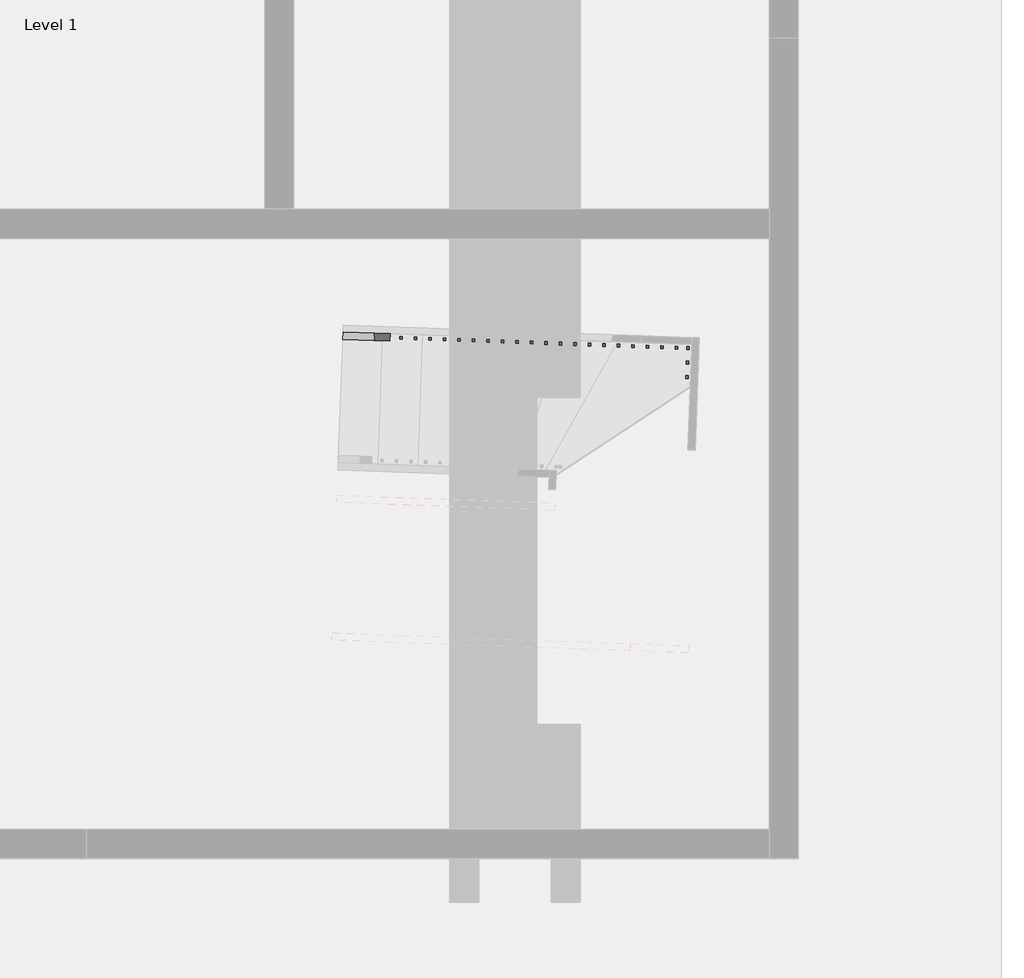
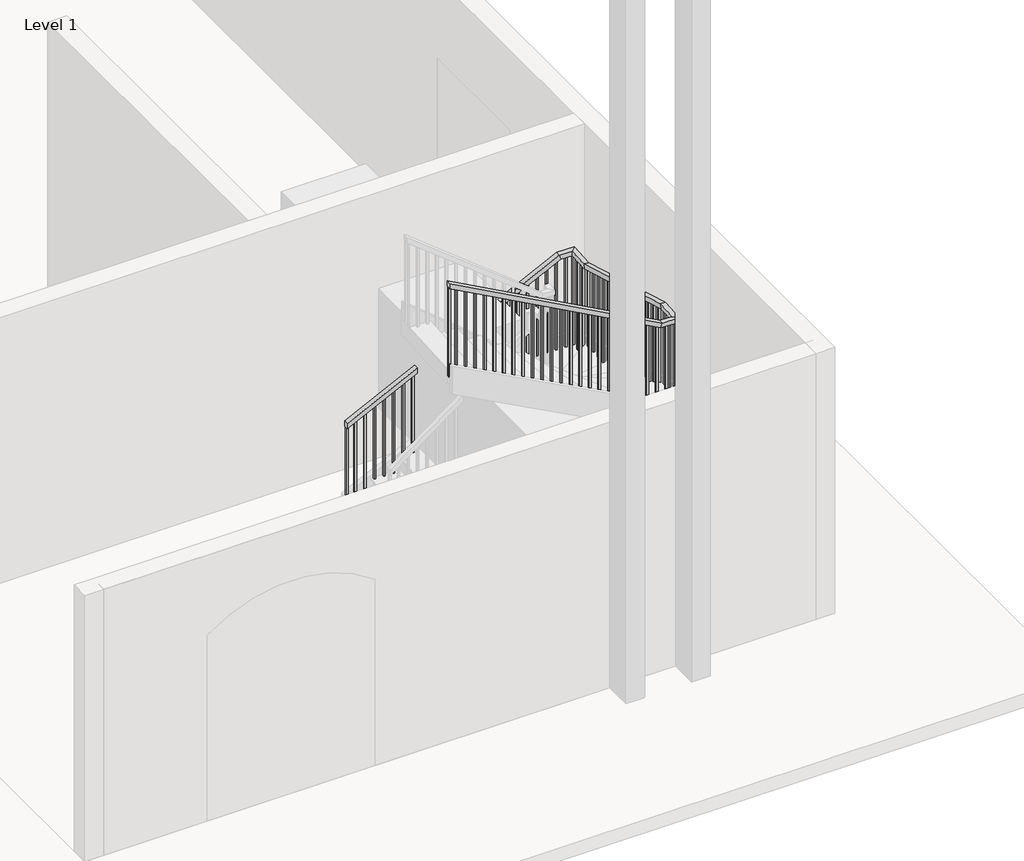
# One storey, part 3 of 4: 1 railing.
"""IFC4 building model written with IfcOpenShell, lengths in millimetres."""

from ifc_helpers import new_model, si_unit, frame, origin, place, context, project, spatial, polyline, outline, extrude, faceted_brep, element, save

model = new_model("IFC4")

# Units and contexts
model_context = context("Model", 3, world=origin())
ifc_project = project(units=[si_unit("LENGTHUNIT", "METRE", prefix="MILLI")], contexts=[model_context])

# Site, building, storey
site = spatial("IfcSite", under=ifc_project)
building = spatial("IfcBuilding", under=site)
storey = spatial("IfcBuildingStorey", under=building, Name="Level 1", Elevation=0.0)

# Railing
placement = place(None, origin())
element("IfcRailing", 1, ObjectType="Handrail - Rectangular", at=placement, inside=storey, context=model_context, shape_type="SolidModel", body=[
    faceted_brep([(-10006.394185, -363.3128759, 1083.7333333), (-10006.394185, -363.3128759, 1026.2742652), (-10008.220866, -414.0800231, 1026.2742652), (-10008.220866, -414.0800231, 1083.7333333), (-7750.1292126, -444.496803, 2277.0239201), (-7737.5382959, -444.9498438, 2226.2239201), (-7739.364977, -495.716991, 2226.2239201), (-7751.9558936, -495.2639503, 2277.0239201), (-7565.8418401, -451.1277497, 2277.0239201), (-7565.8418401, -451.1277497, 2226.2239201), (-7618.4356683, -500.0682159, 2226.2239201), (-7618.4356683, -500.0682159, 2277.0239201), (-7576.1730834, -738.2538248, 2277.0239201), (-7576.4589725, -746.1992592, 2226.2239201), (-7627.2261197, -744.3725782, 2226.2239201), (-7626.9402306, -736.4271438, 2277.0239201), (-7631.3178587, -2270.838284, 2769.1094132), (-7631.6037478, -2278.7837184, 2718.3094132), (-7682.370895, -2276.9570374, 2718.3094132), (-7682.0850059, -2269.011603, 2769.1094132), (-7641.649102, -2557.9643591, 2769.1094132), (-7641.649102, -2557.9643591, 2718.3094132), (-7690.5895682, -2505.3705309, 2718.3094132), (-7690.5895682, -2505.3705309, 2769.1094132), (-7825.9364745, -2551.3334125, 2769.1094132), (-7838.5273911, -2550.8803717, 2718.3094132), (-7836.7007101, -2500.1132245, 2718.3094132), (-7824.1097935, -2500.5662653, 2769.1094132), (-10082.2014469, -2470.1494854, 3962.4), (-10080.3747659, -2419.3823382, 3962.4), (-10080.3747659, -2419.3823382, 3904.9409318), (-10082.2014469, -2470.1494854, 3904.9409318)], [[[0, 1, 2, 3]], [[1, 0, 4, 5]], [[2, 1, 5, 6]], [[3, 2, 6, 7]], [[0, 3, 7, 4]], [[5, 4, 8, 9]], [[6, 5, 9, 10]], [[7, 6, 10, 11]], [[4, 7, 11, 8]], [[9, 8, 12, 13]], [[10, 9, 13, 14]], [[11, 10, 14, 15]], [[8, 11, 15, 12]], [[13, 12, 16, 17]], [[14, 13, 17, 18]], [[15, 14, 18, 19]], [[12, 15, 19, 16]], [[17, 16, 20, 21]], [[18, 17, 21, 22]], [[19, 18, 22, 23]], [[16, 19, 23, 20]], [[21, 20, 24, 25]], [[22, 21, 25, 26]], [[23, 22, 26, 27]], [[20, 23, 27, 24]], [[28, 29, 30, 31]], [[25, 24, 28, 31]], [[26, 25, 31, 30]], [[27, 26, 30, 29]], [[24, 27, 29, 28]]]),
    extrude(outline(polyline([(223.5656878, 19.05), (1212.6274313, 19.05), (1212.6274313, 0.0), (233.6343122, 0.0), (223.5656878, 19.05)])), frame((-9992.2317697, -2457.5014613, 4091.294098), z_axis=(0.035958287618052934, 0.9993532916599503, 0.0), x_axis=(0.0, 0.0, -1.0)), (0.0, 0.0, 1.0), 19.05),
    extrude(outline(polyline([(223.5656878, 19.05), (1158.9281011, 19.05), (1158.9281011, 0.0), (233.6343122, 0.0), (223.5656878, 19.05)])), frame((-9890.6974752, -2461.1548233, 4037.5947678), z_axis=(0.035958287618052934, 0.9993532916599503, 0.0), x_axis=(0.0, 0.0, -1.0)), (0.0, 0.0, 1.0), 19.05),
    extrude(outline(polyline([(223.5656878, 19.05), (1274.5621043, 19.05), (1274.5621043, 0.0), (233.6343122, 0.0), (223.5656878, 19.05)])), frame((-9789.1631808, -2464.8081854, 3983.8954376), z_axis=(0.035958287618052934, 0.9993532916599503, 0.0), x_axis=(0.0, 0.0, -1.0)), (0.0, 0.0, 1.0), 19.05),
    extrude(outline(polyline([(223.5656878, 19.05), (1220.8627741, 19.05), (1220.8627741, 0.0), (233.6343122, 0.0), (223.5656878, 19.05)])), frame((-9687.6288864, -2468.4615474, 3930.1961074), z_axis=(0.035958287618052934, 0.9993532916599503, 0.0), x_axis=(0.0, 0.0, -1.0)), (0.0, 0.0, 1.0), 19.05),
    extrude(outline(polyline([(223.5656878, 19.05), (1167.1634439, 19.05), (1167.1634439, 0.0), (233.6343122, 0.0), (223.5656878, 19.05)])), frame((-9586.0945919, -2472.1149094, 3876.4967772), z_axis=(0.035958287618052934, 0.9993532916599503, 0.0), x_axis=(0.0, 0.0, -1.0)), (0.0, 0.0, 1.0), 19.05),
    extrude(outline(polyline([(223.5656878, 19.05), (1282.797447, 19.05), (1282.797447, 0.0), (233.6343122, 0.0), (223.5656878, 19.05)])), frame((-9484.5602975, -2475.7682714, 3822.797447), z_axis=(0.035958287618052934, 0.9993532916599503, 0.0), x_axis=(0.0, 0.0, -1.0)), (0.0, 0.0, 1.0), 19.05),
    extrude(outline(polyline([(223.5656878, 19.05), (1229.0981168, 19.05), (1229.0981168, 0.0), (233.6343122, 0.0), (223.5656878, 19.05)])), frame((-9383.0260031, -2479.4216334, 3769.0981168), z_axis=(0.035958287618052934, 0.9993532916599503, 0.0), x_axis=(0.0, 0.0, -1.0)), (0.0, 0.0, 1.0), 19.05),
    extrude(outline(polyline([(223.5656878, 19.05), (1175.3987866, 19.05), (1175.3987866, 0.0), (233.6343122, 0.0), (223.5656878, 19.05)])), frame((-9281.4917086, -2483.0749955, 3715.3987866), z_axis=(0.035958287618052934, 0.9993532916599503, 0.0), x_axis=(0.0, 0.0, -1.0)), (0.0, 0.0, 1.0), 19.05),
    extrude(outline(polyline([(223.5656878, 19.05), (1291.0327897, 19.05), (1291.0327897, 0.0), (233.6343122, 0.0), (223.5656878, 19.05)])), frame((-9179.9574142, -2486.7283575, 3661.6994564), z_axis=(0.035958287618052934, 0.9993532916599503, 0.0), x_axis=(0.0, 0.0, -1.0)), (0.0, 0.0, 1.0), 19.05),
    extrude(outline(polyline([(223.5656878, 19.05), (1237.3334595, 19.05), (1237.3334595, 0.0), (233.6343122, 0.0), (223.5656878, 19.05)])), frame((-9078.4231198, -2490.3817195, 3608.0001262), z_axis=(0.035958287618052934, 0.9993532916599503, 0.0), x_axis=(0.0, 0.0, -1.0)), (0.0, 0.0, 1.0), 19.05),
    extrude(outline(polyline([(223.5656878, 19.05), (1183.6341293, 19.05), (1183.6341293, 0.0), (233.6343122, 0.0), (223.5656878, 19.05)])), frame((-8976.8888253, -2494.0350815, 3554.300796), z_axis=(0.035958287618052934, 0.9993532916599503, 0.0), x_axis=(0.0, 0.0, -1.0)), (0.0, 0.0, 1.0), 19.05),
    extrude(outline(polyline([(223.5656878, 19.05), (1299.2681325, 19.05), (1299.2681325, 0.0), (233.6343122, 0.0), (223.5656878, 19.05)])), frame((-8875.3545309, -2497.6884436, 3500.6014658), z_axis=(0.035958287618052934, 0.9993532916599503, 0.0), x_axis=(0.0, 0.0, -1.0)), (0.0, 0.0, 1.0), 19.05),
    extrude(outline(polyline([(223.5656878, 19.05), (1245.5688023, 19.05), (1245.5688023, 0.0), (233.6343122, 0.0), (223.5656878, 19.05)])), frame((-8773.8202365, -2501.3418056, 3446.9021356), z_axis=(0.035958287618052934, 0.9993532916599503, 0.0), x_axis=(0.0, 0.0, -1.0)), (0.0, 0.0, 1.0), 19.05),
    extrude(outline(polyline([(223.5656878, 19.05), (1191.8694721, 19.05), (1191.8694721, 0.0), (233.6343122, 0.0), (223.5656878, 19.05)])), frame((-8672.285942, -2504.9951676, 3393.2028054), z_axis=(0.035958287618052934, 0.9993532916599503, 0.0), x_axis=(0.0, 0.0, -1.0)), (0.0, 0.0, 1.0), 19.05),
    extrude(outline(polyline([(223.5656878, 19.05), (1138.1701419, 19.05), (1138.1701419, 0.0), (233.6343122, 0.0), (223.5656878, 19.05)])), frame((-8570.7516476, -2508.6485296, 3339.5034752), z_axis=(0.035958287618052934, 0.9993532916599503, 0.0), x_axis=(0.0, 0.0, -1.0)), (0.0, 0.0, 1.0), 19.05),
    extrude(outline(polyline([(223.5656878, 19.05), (1253.804145, 19.05), (1253.804145, 0.0), (233.6343122, 0.0), (223.5656878, 19.05)])), frame((-8469.2173532, -2512.3018916, 3285.804145), z_axis=(0.035958287618052934, 0.9993532916599503, 0.0), x_axis=(0.0, 0.0, -1.0)), (0.0, 0.0, 1.0), 19.05),
    extrude(outline(polyline([(223.5656878, 19.05), (1200.1048148, 19.05), (1200.1048148, 0.0), (233.6343122, 0.0), (223.5656878, 19.05)])), frame((-8367.6830587, -2515.9552537, 3232.1048148), z_axis=(0.035958287618052934, 0.9993532916599503, 0.0), x_axis=(0.0, 0.0, -1.0)), (0.0, 0.0, 1.0), 19.05),
    extrude(outline(polyline([(223.5656878, 19.05), (1146.4054846, 19.05), (1146.4054846, 0.0), (233.6343122, 0.0), (223.5656878, 19.05)])), frame((-8266.1487643, -2519.6086157, 3178.4054846), z_axis=(0.035958287618052934, 0.9993532916599503, 0.0), x_axis=(0.0, 0.0, -1.0)), (0.0, 0.0, 1.0), 19.05),
    extrude(outline(polyline([(223.5656878, 19.05), (1092.7061544, 19.05), (1092.7061544, 0.0), (233.6343122, 0.0), (223.5656878, 19.05)])), frame((-8164.6144699, -2523.2619777, 3124.7061544), z_axis=(0.035958287618052934, 0.9993532916599503, 0.0), x_axis=(0.0, 0.0, -1.0)), (0.0, 0.0, 1.0), 19.05),
    extrude(outline(polyline([(223.5656878, 19.05), (1208.3401575, 19.05), (1208.3401575, 0.0), (233.6343122, 0.0), (223.5656878, 19.05)])), frame((-8063.0801754, -2526.9153397, 3071.0068242), z_axis=(0.035958287618052934, 0.9993532916599503, 0.0), x_axis=(0.0, 0.0, -1.0)), (0.0, 0.0, 1.0), 19.05),
    extrude(outline(polyline([(223.5656878, 19.05), (1154.6408273, 19.05), (1154.6408273, 0.0), (233.6343122, 0.0), (223.5656878, 19.05)])), frame((-7961.545881, -2530.5687018, 3017.307494), z_axis=(0.035958287618052934, 0.9993532916599503, 0.0), x_axis=(0.0, 0.0, -1.0)), (0.0, 0.0, 1.0), 19.05),
    extrude(outline(polyline([(223.5656878, 19.05), (1100.9414971, 19.05), (1100.9414971, 0.0), (233.6343122, 0.0), (223.5656878, 19.05)])), frame((-7860.0115866, -2534.2220638, 2963.6081638), z_axis=(0.035958287618052934, 0.9993532916599503, 0.0), x_axis=(0.0, 0.0, -1.0)), (0.0, 0.0, 1.0), 19.05),
    extrude(outline(polyline([(-7758.4772921, -2537.8754258), (-7777.5149723, -2537.1904204), (-7776.829967, -2518.1527402), (-7757.7922868, -2518.8377456), (-7758.4772921, -2537.8754258)])), frame((0.0, 0.0, 1862.6666667), z_axis=(0.0, 0.0, 1.0), x_axis=(1.0, 0.0, 0.0)), (0.0, 0.0, 1.0), 855.6427466),
    extrude(outline(polyline([(-7655.3446518, -2497.107534), (-7656.0296572, -2516.1452142), (-7675.0673374, -2515.4602088), (-7674.382332, -2496.4225286), (-7655.3446518, -2497.107534)])), frame((0.0, 0.0, 1862.6666667), z_axis=(0.0, 0.0, 1.0), x_axis=(1.0, 0.0, 0.0)), (0.0, 0.0, 1.0), 855.6427466),
    extrude(outline(polyline([(-7651.6912898, -2395.5732396), (-7652.3762952, -2414.6109198), (-7671.4139754, -2413.9259144), (-7670.72897, -2394.8882342), (-7651.6912898, -2395.5732396)])), frame((0.0, 0.0, 1862.6666667), z_axis=(0.0, 0.0, 1.0), x_axis=(1.0, 0.0, 0.0)), (0.0, 0.0, 1.0), 855.6427466),
    extrude(outline(polyline([(-7648.0379278, -2294.0389451), (-7648.7229332, -2313.0766254), (-7667.7606134, -2312.39162), (-7667.075608, -2293.3539398), (-7648.0379278, -2294.0389451)])), frame((0.0, 0.0, 1862.6666667), z_axis=(0.0, 0.0, 1.0), x_axis=(1.0, 0.0, 0.0)), (0.0, 0.0, 1.0), 855.6427466),
    extrude(outline(polyline([(225.5436705, 19.05), (1229.1130279, 19.05), (1229.1130279, 0.0), (231.6563296, 0.0), (225.5436705, 19.05)])), frame((-7644.3845658, -2192.5046507, 2922.4463612), z_axis=(-0.9993532916599501, 0.03595828761805307, 0.0), x_axis=(0.0, 0.0, -1.0)), (0.0, 0.0, 1.0), 19.05),
    extrude(outline(polyline([(225.5436704, 19.05), (1196.5121796, 19.05), (1196.5121796, 0.0), (231.6563295, 0.0), (225.5436704, 19.05)])), frame((-7640.7312037, -2090.9703563, 2889.8455129), z_axis=(-0.9993532916599501, 0.03595828761805307, 0.0), x_axis=(0.0, 0.0, -1.0)), (0.0, 0.0, 1.0), 19.05),
    extrude(outline(polyline([(225.5436705, 19.0500001), (1163.9113314, 19.0500001), (1163.9113314, 0.0), (231.6563295, 0.0), (225.5436705, 19.0500001)])), frame((-7637.0778417, -1989.4360618, 2857.2446647), z_axis=(-0.9993532916599501, 0.03595828761805307, 0.0), x_axis=(0.0, 0.0, -1.0)), (0.0, 0.0, 1.0), 19.05),
    extrude(outline(polyline([(225.5436705, 19.05), (1131.3104832, 19.05), (1131.3104832, 0.0), (231.6563295, 0.0), (225.5436705, 19.05)])), frame((-7633.4244797, -1887.9017674, 2824.6438165), z_axis=(-0.9993532916599501, 0.03595828761805307, 0.0), x_axis=(0.0, 0.0, -1.0)), (0.0, 0.0, 1.0), 19.05),
    extrude(outline(polyline([(225.5436705, 19.05), (1098.709635, 19.05), (1098.709635, 0.0), (231.6563296, 0.0), (225.5436705, 19.05)])), frame((-7629.7711177, -1786.367473, 2792.0429683), z_axis=(-0.9993532916599501, 0.03595828761805307, 0.0), x_axis=(0.0, 0.0, -1.0)), (0.0, 0.0, 1.0), 19.05),
    extrude(outline(polyline([(225.5436705, 19.0500001), (1235.44212, 19.0500001), (1235.44212, 0.0), (231.6563295, 0.0), (225.5436705, 19.0500001)])), frame((-7626.1177556, -1684.8331785, 2759.44212), z_axis=(-0.9993532916599501, 0.03595828761805307, 0.0), x_axis=(0.0, 0.0, -1.0)), (0.0, 0.0, 1.0), 19.05),
    extrude(outline(polyline([(225.5436705, 19.05), (1202.8412718, 19.05), (1202.8412718, 0.0), (231.6563295, 0.0), (225.5436705, 19.05)])), frame((-7622.4643936, -1583.2988841, 2726.8412718), z_axis=(-0.9993532916599501, 0.03595828761805307, 0.0), x_axis=(0.0, 0.0, -1.0)), (0.0, 0.0, 1.0), 19.05),
    extrude(outline(polyline([(225.5436705, 19.05), (1170.2404236, 19.05), (1170.2404236, 0.0), (231.6563295, 0.0), (225.5436705, 19.05)])), frame((-7618.8110316, -1481.7645897, 2694.2404236), z_axis=(-0.9993532916599501, 0.03595828761805307, 0.0), x_axis=(0.0, 0.0, -1.0)), (0.0, 0.0, 1.0), 19.05),
    extrude(outline(polyline([(225.5436704, 19.05), (1137.6395753, 19.05), (1137.6395753, 0.0), (231.6563295, 0.0), (225.5436704, 19.05)])), frame((-7615.1576696, -1380.2302953, 2661.6395753), z_axis=(-0.9993532916599501, 0.03595828761805307, 0.0), x_axis=(0.0, 0.0, -1.0)), (0.0, 0.0, 1.0), 19.05),
    extrude(outline(polyline([(225.5436705, 19.05), (1105.0387271, 19.05), (1105.0387271, 0.0), (231.6563295, 0.0), (225.5436705, 19.05)])), frame((-7611.5043076, -1278.6960008, 2629.0387271), z_axis=(-0.9993532916599501, 0.03595828761805307, 0.0), x_axis=(0.0, 0.0, -1.0)), (0.0, 0.0, 1.0), 19.05),
    extrude(outline(polyline([(225.5436705, 19.05), (1241.7712122, 19.05), (1241.7712122, 0.0), (231.6563295, 0.0), (225.5436705, 19.05)])), frame((-7607.8509455, -1177.1617064, 2596.4378789), z_axis=(-0.9993532916599501, 0.03595828761805307, 0.0), x_axis=(0.0, 0.0, -1.0)), (0.0, 0.0, 1.0), 19.05),
    extrude(outline(polyline([(225.5436705, 19.05), (1209.170364, 19.05), (1209.170364, 0.0), (231.6563296, 0.0), (225.5436705, 19.05)])), frame((-7604.1975835, -1075.627412, 2563.8370307), z_axis=(-0.9993532916599501, 0.03595828761805307, 0.0), x_axis=(0.0, 0.0, -1.0)), (0.0, 0.0, 1.0), 19.05),
    extrude(outline(polyline([(225.5436704, 19.05), (1176.5695157, 19.05), (1176.5695157, 0.0), (231.6563295, 0.0), (225.5436704, 19.05)])), frame((-7600.5442215, -974.0931175, 2531.2361824), z_axis=(-0.9993532916599501, 0.03595828761805307, 0.0), x_axis=(0.0, 0.0, -1.0)), (0.0, 0.0, 1.0), 19.05),
    extrude(outline(polyline([(225.5436705, 19.05), (1143.9686675, 19.05), (1143.9686675, 0.0), (231.6563295, 0.0), (225.5436705, 19.05)])), frame((-7596.8908595, -872.5588231, 2498.6353342), z_axis=(-0.9993532916599501, 0.03595828761805307, 0.0), x_axis=(0.0, 0.0, -1.0)), (0.0, 0.0, 1.0), 19.05),
    extrude(outline(polyline([(225.5436705, 19.05), (1111.3678193, 19.05), (1111.3678193, 0.0), (231.6563295, 0.0), (225.5436705, 19.05)])), frame((-7593.2374974, -771.0245287, 2466.034486), z_axis=(-0.9993532916599501, 0.03595828761805307, 0.0), x_axis=(0.0, 0.0, -1.0)), (0.0, 0.0, 1.0), 19.05),
    extrude(outline(polyline([(-7589.5841354, -669.4902342), (-7590.2691408, -688.5279144), (-7609.306821, -687.842909), (-7608.6218156, -668.8052288), (-7589.5841354, -669.4902342)])), frame((0.0, 0.0, 1185.3333333), z_axis=(0.0, 0.0, 1.0), x_axis=(1.0, 0.0, 0.0)), (0.0, 0.0, 1.0), 1040.8905868),
    extrude(outline(polyline([(-7585.9307734, -567.9559398), (-7586.6157788, -586.99362), (-7605.653459, -586.3086146), (-7604.9684536, -567.2709344), (-7585.9307734, -567.9559398)])), frame((0.0, 0.0, 1185.3333333), z_axis=(0.0, 0.0, 1.0), x_axis=(1.0, 0.0, 0.0)), (0.0, 0.0, 1.0), 1040.8905868),
    extrude(outline(polyline([(-7681.195091, -462.8624332), (-7662.1574108, -463.5474386), (-7662.8424161, -482.5851188), (-7681.8800963, -481.9001134), (-7681.195091, -462.8624332)])), frame((0.0, 0.0, 1185.3333333), z_axis=(0.0, 0.0, 1.0), x_axis=(1.0, 0.0, 0.0)), (0.0, 0.0, 1.0), 1040.8905868),
    extrude(outline(polyline([(233.6343122, 19.05), (1250.9261963, 19.05), (1250.9261963, 0.0), (223.5656878, 0.0), (233.6343122, 19.05)])), frame((-7764.3767106, -478.9317568, 2436.2595296), z_axis=(0.03595828761805286, 0.9993532916599503, 0.0), x_axis=(0.0, 0.0, -1.0)), (0.0, 0.0, 1.0), 19.05),
    extrude(outline(polyline([(233.6343122, 19.05), (1197.2268661, 19.05), (1197.2268661, 0.0), (223.5656878, 0.0), (233.6343122, 19.05)])), frame((-7865.911005, -475.2783948, 2382.5601994), z_axis=(0.03595828761805286, 0.9993532916599503, 0.0), x_axis=(0.0, 0.0, -1.0)), (0.0, 0.0, 1.0), 19.05),
    extrude(outline(polyline([(233.6343122, 19.05), (1143.5275359, 19.05), (1143.5275359, 0.0), (223.5656878, 0.0), (233.6343122, 19.05)])), frame((-7967.4452994, -471.6250327, 2328.8608692), z_axis=(0.03595828761805286, 0.9993532916599503, 0.0), x_axis=(0.0, 0.0, -1.0)), (0.0, 0.0, 1.0), 19.05),
    extrude(outline(polyline([(233.6343122, 19.05), (1089.8282057, 19.05), (1089.8282057, 0.0), (223.5656878, 0.0), (233.6343122, 19.05)])), frame((-8068.9795939, -467.9716707, 2275.161539), z_axis=(0.03595828761805286, 0.9993532916599503, 0.0), x_axis=(0.0, 0.0, -1.0)), (0.0, 0.0, 1.0), 19.05),
    extrude(outline(polyline([(233.6343122, 19.05), (1205.4622088, 19.05), (1205.4622088, 0.0), (223.5656878, 0.0), (233.6343122, 19.05)])), frame((-8170.5138883, -464.3183087, 2221.4622088), z_axis=(0.03595828761805286, 0.9993532916599503, 0.0), x_axis=(0.0, 0.0, -1.0)), (0.0, 0.0, 1.0), 19.05),
    extrude(outline(polyline([(233.6343122, 19.05), (1151.7628786, 19.05), (1151.7628786, 0.0), (223.5656878, 0.0), (233.6343122, 19.05)])), frame((-8272.0481827, -460.6649467, 2167.7628786), z_axis=(0.03595828761805286, 0.9993532916599503, 0.0), x_axis=(0.0, 0.0, -1.0)), (0.0, 0.0, 1.0), 19.05),
    extrude(outline(polyline([(233.6343122, 19.05), (1098.0635484, 19.05), (1098.0635484, 0.0), (223.5656878, 0.0), (233.6343122, 19.05)])), frame((-8373.5824772, -457.0115846, 2114.0635484), z_axis=(0.03595828761805286, 0.9993532916599503, 0.0), x_axis=(0.0, 0.0, -1.0)), (0.0, 0.0, 1.0), 19.05),
    extrude(outline(polyline([(233.6343122, 19.05), (1044.3642182, 19.05), (1044.3642182, 0.0), (223.5656878, 0.0), (233.6343122, 19.05)])), frame((-8475.1167716, -453.3582226, 2060.3642182), z_axis=(0.03595828761805286, 0.9993532916599503, 0.0), x_axis=(0.0, 0.0, -1.0)), (0.0, 0.0, 1.0), 19.05),
    extrude(outline(polyline([(233.6343122, 19.05), (1159.9982213, 19.05), (1159.9982213, 0.0), (223.5656878, 0.0), (233.6343122, 19.05)])), frame((-8576.651066, -449.7048606, 2006.664888), z_axis=(0.03595828761805286, 0.9993532916599503, 0.0), x_axis=(0.0, 0.0, -1.0)), (0.0, 0.0, 1.0), 19.05),
    extrude(outline(polyline([(233.6343122, 19.05), (1106.2988911, 19.05), (1106.2988911, 0.0), (223.5656878, 0.0), (233.6343122, 19.05)])), frame((-8678.1853605, -446.0514986, 1952.9655578), z_axis=(0.03595828761805286, 0.9993532916599503, 0.0), x_axis=(0.0, 0.0, -1.0)), (0.0, 0.0, 1.0), 19.05),
    extrude(outline(polyline([(233.6343122, 19.05), (1052.5995609, 19.05), (1052.5995609, 0.0), (223.5656878, 0.0), (233.6343122, 19.05)])), frame((-8779.7196549, -442.3981366, 1899.2662276), z_axis=(0.03595828761805286, 0.9993532916599503, 0.0), x_axis=(0.0, 0.0, -1.0)), (0.0, 0.0, 1.0), 19.05),
    extrude(outline(polyline([(233.6343122, 19.05), (1168.2335641, 19.05), (1168.2335641, 0.0), (223.5656878, 0.0), (233.6343122, 19.05)])), frame((-8881.2539493, -438.7447745, 1845.5668974), z_axis=(0.03595828761805286, 0.9993532916599503, 0.0), x_axis=(0.0, 0.0, -1.0)), (0.0, 0.0, 1.0), 19.05),
    extrude(outline(polyline([(233.6343122, 19.05), (1114.5342339, 19.05), (1114.5342339, 0.0), (223.5656878, 0.0), (233.6343122, 19.05)])), frame((-8982.7882438, -435.0914125, 1791.8675672), z_axis=(0.03595828761805286, 0.9993532916599503, 0.0), x_axis=(0.0, 0.0, -1.0)), (0.0, 0.0, 1.0), 19.05),
    extrude(outline(polyline([(233.6343122, 19.05), (1060.8349037, 19.05), (1060.8349037, 0.0), (223.5656878, 0.0), (233.6343122, 19.05)])), frame((-9084.3225382, -431.4380505, 1738.168237), z_axis=(0.03595828761805286, 0.9993532916599503, 0.0), x_axis=(0.0, 0.0, -1.0)), (0.0, 0.0, 1.0), 19.05),
    extrude(outline(polyline([(233.6343122, 19.05), (1176.4689068, 19.05), (1176.4689068, 0.0), (223.5656878, 0.0), (233.6343122, 19.05)])), frame((-9185.8568326, -427.7846885, 1684.4689068), z_axis=(0.03595828761805286, 0.9993532916599503, 0.0), x_axis=(0.0, 0.0, -1.0)), (0.0, 0.0, 1.0), 19.05),
    extrude(outline(polyline([(233.6343122, 19.05), (1122.7695766, 19.05), (1122.7695766, 0.0), (223.5656878, 0.0), (233.6343122, 19.05)])), frame((-9287.3911271, -424.1313264, 1630.7695766), z_axis=(0.03595828761805286, 0.9993532916599503, 0.0), x_axis=(0.0, 0.0, -1.0)), (0.0, 0.0, 1.0), 19.05),
    extrude(outline(polyline([(233.6343122, 19.05), (1069.0702464, 19.05), (1069.0702464, 0.0), (223.5656878, 0.0), (233.6343122, 19.05)])), frame((-9388.9254215, -420.4779644, 1577.0702464), z_axis=(0.03595828761805286, 0.9993532916599503, 0.0), x_axis=(0.0, 0.0, -1.0)), (0.0, 0.0, 1.0), 19.05),
    extrude(outline(polyline([(233.6343122, 19.05), (1184.7042495, 19.05), (1184.7042495, 0.0), (223.5656878, 0.0), (233.6343122, 19.05)])), frame((-9490.4597159, -416.8246024, 1523.3709162), z_axis=(0.03595828761805286, 0.9993532916599503, 0.0), x_axis=(0.0, 0.0, -1.0)), (0.0, 0.0, 1.0), 19.05),
    extrude(outline(polyline([(233.6343122, 19.05), (1131.0049193, 19.05), (1131.0049193, 0.0), (223.5656878, 0.0), (233.6343122, 19.05)])), frame((-9591.9940104, -413.1712404, 1469.671586), z_axis=(0.03595828761805286, 0.9993532916599503, 0.0), x_axis=(0.0, 0.0, -1.0)), (0.0, 0.0, 1.0), 19.05),
    extrude(outline(polyline([(233.6343122, 19.05), (1077.3055891, 19.05), (1077.3055891, 0.0), (223.5656878, 0.0), (233.6343122, 19.05)])), frame((-9693.5283048, -409.5178784, 1415.9722558), z_axis=(0.03595828761805286, 0.9993532916599503, 0.0), x_axis=(0.0, 0.0, -1.0)), (0.0, 0.0, 1.0), 19.05),
    extrude(outline(polyline([(233.6343122, 19.05), (1192.9395923, 19.05), (1192.9395923, 0.0), (223.5656878, 0.0), (233.6343122, 19.05)])), frame((-9795.0625992, -405.8645163, 1362.2729256), z_axis=(0.03595828761805286, 0.9993532916599503, 0.0), x_axis=(0.0, 0.0, -1.0)), (0.0, 0.0, 1.0), 19.05),
    extrude(outline(polyline([(233.6343123, 19.0500001), (1139.2402621, 19.0500001), (1139.2402621, 0.0), (223.5656878, 0.0), (233.6343123, 19.0500001)])), frame((-9896.5968936, -402.2111543, 1308.5735954), z_axis=(0.03595828761805286, 0.9993532916599503, 0.0), x_axis=(0.0, 0.0, -1.0)), (0.0, 0.0, 1.0), 19.05),
    extrude(outline(polyline([(-7656.2579923, -2522.4911076), (-7656.9429977, -2541.5287878), (-7675.9806779, -2540.8437824), (-7675.2956725, -2521.8061022), (-7656.2579923, -2522.4911076)])), frame((0.0, 0.0, 1862.6666667), z_axis=(0.0, 0.0, 1.0), x_axis=(1.0, 0.0, 0.0)), (0.0, 0.0, 1.0), 855.6427466),
    extrude(outline(polyline([(-7601.3150916, -465.73664), (-7582.2774114, -466.4216454), (-7582.9624168, -485.4593256), (-7602.000097, -484.7743202), (-7601.3150916, -465.73664)])), frame((0.0, 0.0, 1185.3333333), z_axis=(0.0, 0.0, 1.0), x_axis=(1.0, 0.0, 0.0)), (0.0, 0.0, 1.0), 1040.8905868),
    extrude(outline(polyline([(223.5656878, 19.05), (1249.8399529, 19.05), (1249.8399529, 0.0), (233.6343122, 0.0), (223.5656878, 19.05)])), frame((-10062.5929289, -2454.9697572, 4128.5066196), z_axis=(0.035958287618052934, 0.9993532916599503, 0.0), x_axis=(0.0, 0.0, -1.0)), (0.0, 0.0, 1.0), 19.05),
    extrude(outline(polyline([(233.6343122, 19.05), (1090.5752441, 19.05), (1090.5752441, 0.0), (223.5656878, 0.0), (233.6343122, 19.05)])), frame((-9988.612348, -398.900295, 1259.9085774), z_axis=(0.03595828761805286, 0.9993532916599503, 0.0), x_axis=(0.0, 0.0, -1.0)), (0.0, 0.0, 1.0), 19.05),
])

save(model, "model.ifc")

# Revit data of these elements
# Type "Handrail - Rectangular"
#   Assembly Code = "C2010400"
#   built-in parameter 1008612 = 0.0416667 (stored number, unit not read)
#   built-in parameter 1008611 = 0.0416667 (stored number, unit not read)
#   built-in parameter 1008609 = 0.333333 (stored number, unit not read)
#   built-in parameter 1008604 = 0.166667 (stored number, unit not read)
#   built-in parameter 1008603 = 0.166667 (stored number, unit not read)
#   Railing Height = 3' - 0"
#   built-in parameter 1008630 = 2
#   built-in parameter 1008610 = 2
#   built-in parameter 1008618 = Baluster - Square : 3/4"
# Element 1 (IfcRailing, "Handrail - Rectangular")
#   Phase Created = New Construction
